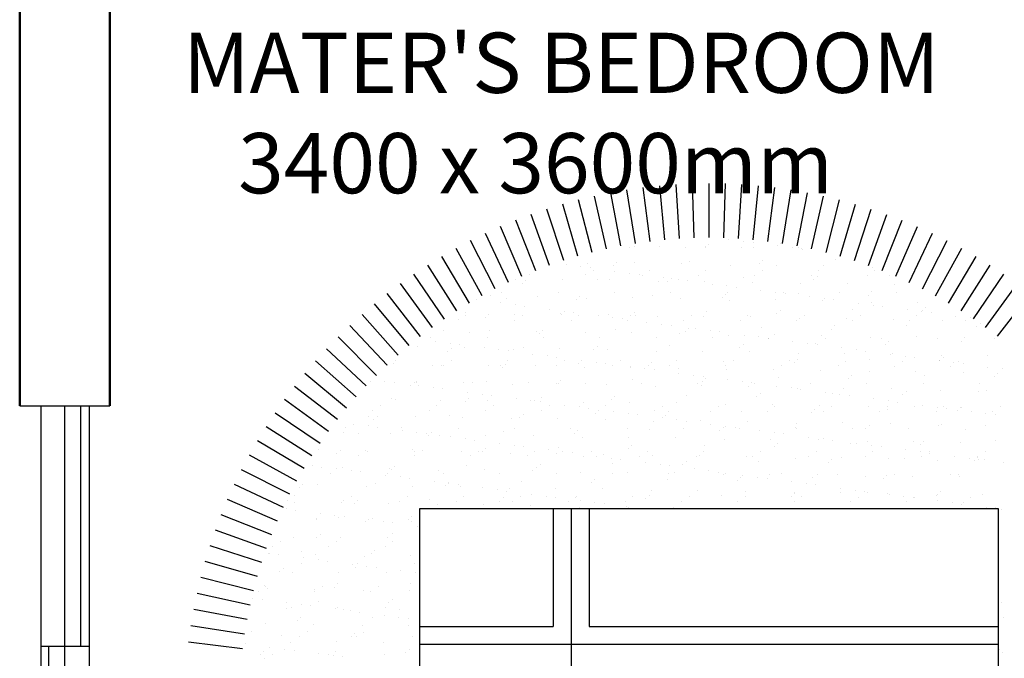
# Model space of a CAD drawing. Units: millimetres. Extents: x -857 to 54106, y -13666 to 13947.
# Tile 14 of 41: x 21020 to 23479, y 5837 to 7433. Entities that reach past the tile are written whole.
import ezdxf

# ---------------------------------------------------------------- set-up
doc = ezdxf.new("R2010")
doc.units = ezdxf.units.MM
for name, color, linetype, lineweight in [('A-AREA-IDEN', 3, 'Continuous', 18), ('A-FURN', 21, 'Continuous', 18), ('A-GLAZ', 4, 'Continuous', 25), ('A-WALL', 7, 'Continuous', 50)]:
    doc.layers.add(name, color=color, linetype=linetype, lineweight=lineweight)
for name, color, linetype in [('A-FRN', 11, 'Continuous'), ('A-HT', 15, 'Continuous'), ('L-HT', 1, 'Continuous')]:
    doc.layers.add(name, color=color, linetype=linetype)
doc.styles.get("Standard").update_dxf_attribs({"font": 'arial.ttf'})

# ---------------------------------------------------------------- blocks, each defined once
blk = doc.blocks.new('*X18')
at = {"color": 0}
for p, q in [((1.8017, 2.833), (1.8017, 2.833)), ((1.8783, 2.8364), (1.8783, 2.8364)), ((1.9044, 2.8399), (1.9044, 2.8399)), ((1.945, 2.8452), (1.945, 2.8452)), ((2.0018, 2.8313), (2.0018, 2.8313)), ((1.7428, 2.8186), (1.7428, 2.8186)), ((1.7438, 2.8187), (1.7438, 2.8187)), ((1.7537, 2.8227), (1.7537, 2.8227)), ((1.7698, 2.8221), (1.7698, 2.8221)), ((1.8104, 2.8275), (1.8104, 2.8275)), ((1.8778, 2.8235), (1.8778, 2.8235)), ((1.9094, 2.823), (1.9094, 2.823)), ((2.0087, 2.8252), (2.0087, 2.8252)), ((2.011, 2.8229), (2.011, 2.8229)), ((2.0652, 2.8233), (2.0652, 2.8233)), ((2.1366, 2.8246), (2.1366, 2.8246)), ((2.2048, 2.8269), (2.2048, 2.8269)), ((2.2209, 2.8236), (2.2209, 2.8236)), ((1.6514, 2.7891), (1.6514, 2.7891)), ((1.8515, 2.7874), (1.8515, 2.7874)), ((1.8607, 2.779), (1.8607, 2.779)), ((2.0545, 2.783), (2.0545, 2.783)), ((2.0763, 2.7783), (2.0763, 2.7783)), ((2.2072, 2.78), (2.2072, 2.78)), ((2.2546, 2.7813), (2.2546, 2.7813)), ((2.3351, 2.7793), (2.3351, 2.7793)), ((1.5414, 2.759), (1.5414, 2.759)), ((1.5474, 2.7675), (1.5474, 2.7675)), ((1.6825, 2.7724), (1.6825, 2.7724)), ((1.6971, 2.7593), (1.6971, 2.7593)), ((1.8133, 2.774), (1.8133, 2.774)), ((1.8528, 2.7596), (1.8528, 2.7596)), ((1.9412, 2.7734), (1.9412, 2.7734)), ((2.0085, 2.7599), (2.0085, 2.7599)), ((2.1643, 2.7602), (2.1643, 2.7602)), ((2.2196, 2.7519), (2.2196, 2.7519)), ((2.2603, 2.7573), (2.2603, 2.7573)), ((2.2638, 2.7728), (2.2638, 2.7728)), ((2.32, 2.7605), (2.32, 2.7605)), ((2.3282, 2.7662), (2.3282, 2.7662)), ((2.3542, 2.7696), (2.3542, 2.7696)), ((2.3949, 2.775), (2.3949, 2.775)), ((1.5011, 2.7453), (1.5011, 2.7453)), ((1.5625, 2.7456), (1.5625, 2.7456)), ((1.618, 2.7229), (1.618, 2.7229)), ((1.7012, 2.7435), (1.7012, 2.7435)), ((1.7104, 2.7351), (1.7104, 2.7351)), ((1.7182, 2.7459), (1.7182, 2.7459)), ((1.7459, 2.7223), (1.7459, 2.7223)), ((1.8739, 2.7462), (1.8739, 2.7462)), ((1.881, 2.7272), (1.881, 2.7272)), ((1.9042, 2.7391), (1.9042, 2.7391)), ((1.9911, 2.7218), (1.9911, 2.7218)), ((2.0118, 2.7288), (2.0118, 2.7288)), ((2.0296, 2.7465), (2.0296, 2.7465)), ((2.059, 2.7308), (2.059, 2.7308)), ((2.0851, 2.7342), (2.0851, 2.7342)), ((2.1043, 2.7374), (2.1043, 2.7374)), ((2.1135, 2.729), (2.1135, 2.729)), ((2.1257, 2.7395), (2.1257, 2.7395)), ((2.1397, 2.7282), (2.1397, 2.7282)), ((2.1853, 2.7467), (2.1853, 2.7467)), ((2.1936, 2.7485), (2.1936, 2.7485)), ((2.2748, 2.7331), (2.2748, 2.7331)), ((2.3073, 2.733), (2.3073, 2.733)), ((2.341, 2.747), (2.341, 2.747)), ((2.4057, 2.7348), (2.4057, 2.7348)), ((2.4967, 2.7473), (2.4967, 2.7473)), ((2.5074, 2.7313), (2.5074, 2.7313)), ((2.5166, 2.7228), (2.5166, 2.7228)), ((2.5336, 2.7341), (2.5336, 2.7341)), ((1.4827, 2.697), (1.4827, 2.697)), ((1.4871, 2.7212), (1.4871, 2.7212)), ((1.5509, 2.6997), (1.5509, 2.6997)), ((1.6384, 2.6973), (1.6384, 2.6973)), ((1.7539, 2.6952), (1.7539, 2.6952)), ((1.7899, 2.6953), (1.7899, 2.6953)), ((1.7941, 2.6975), (1.7941, 2.6975)), ((1.8159, 2.6988), (1.8159, 2.6988)), ((1.8565, 2.7041), (1.8565, 2.7041)), ((1.9244, 2.7131), (1.9244, 2.7131)), ((1.9498, 2.6978), (1.9498, 2.6978)), ((1.9505, 2.7165), (1.9505, 2.7165)), ((2.1055, 2.6981), (2.1055, 2.6981)), ((2.2612, 2.6984), (2.2612, 2.6984)), ((2.4169, 2.6987), (2.4169, 2.6987)), ((2.5727, 2.6989), (2.5727, 2.6989)), ((1.4227, 2.6718), (1.4227, 2.6718)), ((1.5506, 2.6712), (1.5506, 2.6712)), ((1.5601, 2.6912), (1.5601, 2.6912)), ((1.5873, 2.6687), (1.5873, 2.6687)), ((1.6553, 2.6776), (1.6553, 2.6776)), ((1.6813, 2.681), (1.6813, 2.681)), ((1.6856, 2.676), (1.6856, 2.676)), ((1.7219, 2.6864), (1.7219, 2.6864)), ((1.8165, 2.6777), (1.8165, 2.6777)), ((1.9444, 2.6771), (1.9444, 2.6771)), ((1.954, 2.6935), (1.954, 2.6935)), ((1.9632, 2.6851), (1.9632, 2.6851)), ((2.0794, 2.682), (2.0794, 2.682)), ((2.157, 2.6891), (2.157, 2.6891)), ((2.2103, 2.6836), (2.2103, 2.6836)), ((2.3382, 2.683), (2.3382, 2.683)), ((2.3571, 2.6874), (2.3571, 2.6874)), ((2.3663, 2.6789), (2.3663, 2.6789)), ((2.4733, 2.6879), (2.4733, 2.6879)), ((2.5601, 2.683), (2.5601, 2.683)), ((2.5756, 2.6693), (2.5756, 2.6693)), ((2.6042, 2.6895), (2.6042, 2.6895)), ((2.6435, 2.6783), (2.6435, 2.6783)), ((1.3861, 2.6422), (1.3861, 2.6422)), ((1.4006, 2.6558), (1.4006, 2.6558)), ((1.4098, 2.6473), (1.4098, 2.6473)), ((1.4121, 2.6456), (1.4121, 2.6456)), ((1.4528, 2.651), (1.4528, 2.651)), ((1.5207, 2.6599), (1.5207, 2.6599)), ((1.5467, 2.6633), (1.5467, 2.6633)), ((1.6036, 2.6513), (1.6036, 2.6513)), ((1.8037, 2.6496), (1.8037, 2.6496)), ((1.8129, 2.6412), (1.8129, 2.6412)), ((2.0067, 2.6452), (2.0067, 2.6452)), ((2.2068, 2.6435), (2.2068, 2.6435)), ((2.3743, 2.6428), (2.3743, 2.6428)), ((2.4003, 2.6462), (2.4003, 2.6462)), ((2.441, 2.6516), (2.441, 2.6516)), ((2.5089, 2.6605), (2.5089, 2.6605)), ((2.5349, 2.664), (2.5349, 2.664)), ((2.6718, 2.6427), (2.6718, 2.6427)), ((1.2775, 2.6279), (1.2775, 2.6279)), ((1.2915, 2.6198), (1.2915, 2.6198)), ((1.3182, 2.6332), (1.3182, 2.6332)), ((1.3552, 2.62), (1.3552, 2.62)), ((1.4261, 2.6336), (1.4261, 2.6336)), ((1.4472, 2.6201), (1.4472, 2.6201)), ((1.4903, 2.6249), (1.4903, 2.6249)), ((1.5818, 2.6338), (1.5818, 2.6338)), ((1.6029, 2.6204), (1.6029, 2.6204)), ((1.6212, 2.6266), (1.6212, 2.6266)), ((1.7375, 2.6341), (1.7375, 2.6341)), ((1.7491, 2.626), (1.7491, 2.626)), ((1.7586, 2.6207), (1.7586, 2.6207)), ((1.8841, 2.6308), (1.8841, 2.6308)), ((1.8932, 2.6344), (1.8932, 2.6344)), ((1.9143, 2.621), (1.9143, 2.621)), ((2.015, 2.6325), (2.015, 2.6325)), ((2.0489, 2.6347), (2.0489, 2.6347)), ((2.07, 2.6213), (2.07, 2.6213)), ((2.1429, 2.6319), (2.1429, 2.6319)), ((2.1718, 2.6162), (2.1718, 2.6162)), ((2.2046, 2.635), (2.2046, 2.635)), ((2.216, 2.635), (2.216, 2.635)), ((2.2257, 2.6215), (2.2257, 2.6215)), ((2.2397, 2.6251), (2.2397, 2.6251)), ((2.2657, 2.6285), (2.2657, 2.6285)), ((2.2779, 2.6367), (2.2779, 2.6367)), ((2.3064, 2.6339), (2.3064, 2.6339)), ((2.3603, 2.6352), (2.3603, 2.6352)), ((2.3814, 2.6218), (2.3814, 2.6218)), ((2.4088, 2.6384), (2.4088, 2.6384)), ((2.4098, 2.6391), (2.4098, 2.6391)), ((2.516, 2.6355), (2.516, 2.6355)), ((2.5367, 2.6378), (2.5367, 2.6378)), ((2.5371, 2.6221), (2.5371, 2.6221)), ((2.6099, 2.6374), (2.6099, 2.6374)), ((2.6191, 2.6289), (2.6191, 2.6289)), ((2.6718, 2.6358), (2.6718, 2.6358)), ((2.6928, 2.6224), (2.6928, 2.6224)), ((1.2503, 2.6119), (1.2503, 2.6119)), ((1.2595, 2.6034), (1.2595, 2.6034)), ((1.4533, 2.6075), (1.4533, 2.6075)), ((1.6534, 2.6057), (1.6534, 2.6057)), ((1.6626, 2.5973), (1.6626, 2.5973)), ((1.8564, 2.6013), (1.8564, 2.6013)), ((1.9705, 2.5897), (1.9705, 2.5897)), ((1.9966, 2.5931), (1.9966, 2.5931)), ((2.0372, 2.5984), (2.0372, 2.5984)), ((2.0565, 2.5996), (2.0565, 2.5996)), ((2.0657, 2.5912), (2.0657, 2.5912)), ((2.0826, 2.5856), (2.0826, 2.5856)), ((2.1051, 2.6074), (2.1051, 2.6074)), ((2.1312, 2.6108), (2.1312, 2.6108)), ((2.2135, 2.5873), (2.2135, 2.5873)), ((2.2595, 2.5952), (2.2595, 2.5952)), ((2.3414, 2.5867), (2.3414, 2.5867)), ((2.4595, 2.5935), (2.4595, 2.5935)), ((2.4764, 2.5915), (2.4764, 2.5915)), ((2.6073, 2.5932), (2.6073, 2.5932)), ((2.6626, 2.589), (2.6626, 2.589)), ((2.7352, 2.5926), (2.7352, 2.5926)), ((1.2117, 2.5712), (1.2117, 2.5712)), ((1.2949, 2.5738), (1.2949, 2.5738)), ((1.303, 2.5636), (1.303, 2.5636)), ((1.3674, 2.5715), (1.3674, 2.5715)), ((1.4258, 2.5754), (1.4258, 2.5754)), ((1.5031, 2.5619), (1.5031, 2.5619)), ((1.5231, 2.5718), (1.5231, 2.5718)), ((1.5537, 2.5748), (1.5537, 2.5748)), ((1.6788, 2.572), (1.6788, 2.572)), ((1.6888, 2.5797), (1.6888, 2.5797)), ((1.768, 2.563), (1.768, 2.563)), ((1.8196, 2.5814), (1.8196, 2.5814)), ((1.8345, 2.5723), (1.8345, 2.5723)), ((1.836, 2.5719), (1.836, 2.5719)), ((1.862, 2.5754), (1.862, 2.5754)), ((1.9026, 2.5807), (1.9026, 2.5807)), ((1.9475, 2.5807), (1.9475, 2.5807)), ((1.9902, 2.5726), (1.9902, 2.5726)), ((2.1459, 2.5729), (2.1459, 2.5729)), ((2.3016, 2.5732), (2.3016, 2.5732)), ((2.4573, 2.5735), (2.4573, 2.5735)), ((2.4688, 2.585), (2.4688, 2.585)), ((2.613, 2.5737), (2.613, 2.5737)), ((2.7156, 2.5583), (2.7156, 2.5583)), ((2.7563, 2.5636), (2.7563, 2.5636)), ((2.7687, 2.574), (2.7687, 2.574)), ((1.5123, 2.5534), (1.5123, 2.5534)), ((1.5668, 2.5365), (1.5668, 2.5365)), ((1.5928, 2.5399), (1.5928, 2.5399)), ((1.6334, 2.5453), (1.6334, 2.5453)), ((1.7014, 2.5542), (1.7014, 2.5542)), ((1.7061, 2.5574), (1.7061, 2.5574)), ((1.7274, 2.5577), (1.7274, 2.5577)), ((1.8873, 2.5345), (1.8873, 2.5345)), ((1.9061, 2.5557), (1.9061, 2.5557)), ((1.9154, 2.5473), (1.9154, 2.5473)), ((2.0181, 2.5361), (2.0181, 2.5361)), ((2.1092, 2.5513), (2.1092, 2.5513)), ((2.146, 2.5355), (2.146, 2.5355)), ((2.2811, 2.5404), (2.2811, 2.5404)), ((2.3092, 2.5496), (2.3092, 2.5496)), ((2.3185, 2.5411), (2.3185, 2.5411)), ((2.412, 2.5421), (2.412, 2.5421)), ((2.5123, 2.5452), (2.5123, 2.5452)), ((2.5399, 2.5415), (2.5399, 2.5415)), ((2.555, 2.5371), (2.555, 2.5371)), ((2.581, 2.5406), (2.581, 2.5406)), ((2.6217, 2.5459), (2.6217, 2.5459)), ((2.6749, 2.5463), (2.6749, 2.5463)), ((2.6896, 2.5549), (2.6896, 2.5549)), ((2.7123, 2.5434), (2.7123, 2.5434)), ((2.7216, 2.535), (2.7216, 2.535)), ((2.8058, 2.548), (2.8058, 2.548)), ((1.2305, 2.5243), (1.2305, 2.5243)), ((1.3108, 2.5081), (1.3108, 2.5081)), ((1.3236, 2.5045), (1.3236, 2.5045)), ((1.3527, 2.518), (1.3527, 2.518)), ((1.3584, 2.5237), (1.3584, 2.5237)), ((1.362, 2.5095), (1.362, 2.5095)), ((1.3643, 2.5098), (1.3643, 2.5098)), ((1.4322, 2.5188), (1.4322, 2.5188)), ((1.4582, 2.5222), (1.4582, 2.5222)), ((1.4665, 2.5083), (1.4665, 2.5083)), ((1.4934, 2.5286), (1.4934, 2.5286)), ((1.4989, 2.5276), (1.4989, 2.5276)), ((1.5558, 2.5136), (1.5558, 2.5136)), ((1.6222, 2.5086), (1.6222, 2.5086)), ((1.6243, 2.5302), (1.6243, 2.5302)), ((1.7522, 2.5296), (1.7522, 2.5296)), ((1.7558, 2.5118), (1.7558, 2.5118)), ((1.7779, 2.5089), (1.7779, 2.5089)), ((1.9336, 2.5092), (1.9336, 2.5092)), ((1.9589, 2.5074), (1.9589, 2.5074)), ((2.0893, 2.5095), (2.0893, 2.5095)), ((2.1589, 2.5057), (2.1589, 2.5057)), ((2.245, 2.5098), (2.245, 2.5098)), ((2.3118, 2.5051), (2.3118, 2.5051)), ((2.3525, 2.5105), (2.3525, 2.5105)), ((2.4007, 2.51), (2.4007, 2.51)), ((2.4204, 2.5194), (2.4204, 2.5194)), ((2.4464, 2.5229), (2.4464, 2.5229)), ((2.4871, 2.5282), (2.4871, 2.5282)), ((2.5564, 2.5103), (2.5564, 2.5103)), ((2.7121, 2.5106), (2.7121, 2.5106)), ((2.8678, 2.5109), (2.8678, 2.5109)), ((1.189, 2.4868), (1.189, 2.4868)), ((1.2297, 2.4921), (1.2297, 2.4921)), ((1.2976, 2.5011), (1.2976, 2.5011)), ((1.2981, 2.4774), (1.2981, 2.4774)), ((1.3319, 2.4946), (1.3319, 2.4946)), ((1.429, 2.4791), (1.429, 2.4791)), ((1.4876, 2.4949), (1.4876, 2.4949)), ((1.5569, 2.4785), (1.5569, 2.4785)), ((1.6433, 2.4952), (1.6433, 2.4952)), ((1.6919, 2.4833), (1.6919, 2.4833)), ((1.7651, 2.5034), (1.7651, 2.5034)), ((1.799, 2.4955), (1.799, 2.4955)), ((1.8228, 2.485), (1.8228, 2.485)), ((1.9507, 2.4844), (1.9507, 2.4844)), ((1.9547, 2.4958), (1.9547, 2.4958)), ((2.0857, 2.4893), (2.0857, 2.4893)), ((2.1104, 2.496), (2.1104, 2.496)), ((2.1512, 2.484), (2.1512, 2.484)), ((2.1682, 2.4973), (2.1682, 2.4973)), ((2.1773, 2.4874), (2.1773, 2.4874)), ((2.2166, 2.4909), (2.2166, 2.4909)), ((2.2179, 2.4928), (2.2179, 2.4928)), ((2.2661, 2.4963), (2.2661, 2.4963)), ((2.2858, 2.5017), (2.2858, 2.5017)), ((2.3445, 2.4903), (2.3445, 2.4903)), ((2.362, 2.5013), (2.362, 2.5013)), ((2.4218, 2.4966), (2.4218, 2.4966)), ((2.4796, 2.4952), (2.4796, 2.4952)), ((2.562, 2.4996), (2.562, 2.4996)), ((2.5712, 2.4911), (2.5712, 2.4911)), ((2.5775, 2.4969), (2.5775, 2.4969)), ((2.6104, 2.4969), (2.6104, 2.4969)), ((2.7332, 2.4972), (2.7332, 2.4972)), ((2.7384, 2.4962), (2.7384, 2.4962)), ((2.7651, 2.4951), (2.7651, 2.4951)), ((2.8734, 2.5011), (2.8734, 2.5011)), ((2.8889, 2.4975), (2.8889, 2.4975)), ((1.2024, 2.4741), (1.2024, 2.4741)), ((1.2117, 2.4657), (1.2117, 2.4657)), ((1.4055, 2.4697), (1.4055, 2.4697)), ((1.6055, 2.468), (1.6055, 2.468)), ((1.6148, 2.4595), (1.6148, 2.4595)), ((1.8086, 2.4635), (1.8086, 2.4635)), ((1.9081, 2.452), (1.9081, 2.452)), ((1.9487, 2.4573), (1.9487, 2.4573)), ((2.0086, 2.4618), (2.0086, 2.4618)), ((2.0166, 2.4663), (2.0166, 2.4663)), ((2.0178, 2.4534), (2.0178, 2.4534)), ((2.0427, 2.4697), (2.0427, 2.4697)), ((2.0833, 2.4751), (2.0833, 2.4751)), ((2.2117, 2.4574), (2.2117, 2.4574)), ((2.4117, 2.4557), (2.4117, 2.4557)), ((2.6147, 2.4513), (2.6147, 2.4513)), ((2.6781, 2.45), (2.6781, 2.45)), ((2.8089, 2.4516), (2.8089, 2.4516)), ((2.8148, 2.4495), (2.8148, 2.4495)), ((2.8963, 2.4526), (2.8963, 2.4526)), ((2.9368, 2.451), (2.9368, 2.451)), ((1.2336, 2.428), (1.2336, 2.428)), ((1.2521, 2.446), (1.2521, 2.446)), ((1.2552, 2.4258), (1.2552, 2.4258)), ((1.3615, 2.4273), (1.3615, 2.4273)), ((1.4078, 2.4463), (1.4078, 2.4463)), ((1.4552, 2.4241), (1.4552, 2.4241)), ((1.4966, 2.4322), (1.4966, 2.4322)), ((1.5635, 2.4466), (1.5635, 2.4466)), ((1.6275, 2.4339), (1.6275, 2.4339)), ((1.7192, 2.4468), (1.7192, 2.4468)), ((1.7475, 2.4308), (1.7475, 2.4308)), ((1.7554, 2.4333), (1.7554, 2.4333)), ((1.7735, 2.4343), (1.7735, 2.4343)), ((1.8141, 2.4396), (1.8141, 2.4396)), ((1.8749, 2.4471), (1.8749, 2.4471)), ((1.8821, 2.4486), (1.8821, 2.4486)), ((1.8904, 2.4381), (1.8904, 2.4381)), ((2.0213, 2.4398), (2.0213, 2.4398)), ((2.0306, 2.4474), (2.0306, 2.4474)), ((2.1492, 2.4392), (2.1492, 2.4392)), ((2.1863, 2.4477), (2.1863, 2.4477)), ((2.2842, 2.4441), (2.2842, 2.4441)), ((2.342, 2.448), (2.342, 2.448)), ((2.4151, 2.4457), (2.4151, 2.4457)), ((2.4209, 2.4472), (2.4209, 2.4472)), ((2.4977, 2.4483), (2.4977, 2.4483)), ((2.543, 2.4451), (2.543, 2.4451)), ((2.6534, 2.4485), (2.6534, 2.4485)), ((2.6678, 2.4225), (2.6678, 2.4225)), ((2.7357, 2.4315), (2.7357, 2.4315)), ((2.7617, 2.4349), (2.7617, 2.4349)), ((2.8024, 2.4403), (2.8024, 2.4403)), ((2.8091, 2.4488), (2.8091, 2.4488)), ((2.824, 2.4411), (2.824, 2.4411)), ((2.8703, 2.4492), (2.8703, 2.4492)), ((1.4644, 2.4156), (1.4644, 2.4156)), ((1.4783, 2.3954), (1.4783, 2.3954)), ((1.5043, 2.3988), (1.5043, 2.3988)), ((1.545, 2.4042), (1.545, 2.4042)), ((1.6129, 2.4131), (1.6129, 2.4131)), ((1.6389, 2.4165), (1.6389, 2.4165)), ((1.6582, 2.4197), (1.6582, 2.4197)), ((1.6795, 2.4219), (1.6795, 2.4219)), ((1.8583, 2.4179), (1.8583, 2.4179)), ((1.8675, 2.4095), (1.8675, 2.4095)), ((2.0613, 2.4135), (2.0613, 2.4135)), ((2.2614, 2.4118), (2.2614, 2.4118)), ((2.2706, 2.4033), (2.2706, 2.4033)), ((2.4644, 2.4074), (2.4644, 2.4074)), ((2.4665, 2.396), (2.4665, 2.396)), ((2.4827, 2.3988), (2.4827, 2.3988)), ((2.4925, 2.3995), (2.4925, 2.3995)), ((2.5332, 2.4048), (2.5332, 2.4048)), ((2.6011, 2.4138), (2.6011, 2.4138)), ((2.6136, 2.4005), (2.6136, 2.4005)), ((2.6271, 2.4172), (2.6271, 2.4172)), ((2.6645, 2.4057), (2.6645, 2.4057)), ((2.6737, 2.3972), (2.6737, 2.3972)), ((2.7415, 2.3999), (2.7415, 2.3999)), ((2.8675, 2.4012), (2.8675, 2.4012)), ((2.8765, 2.4048), (2.8765, 2.4048)), ((1.1954, 2.3826), (1.1954, 2.3826)), ((1.2165, 2.3691), (1.2165, 2.3691)), ((1.2758, 2.3687), (1.2758, 2.3687)), ((1.3012, 2.3811), (1.3012, 2.3811)), ((1.3049, 2.3802), (1.3049, 2.3802)), ((1.3141, 2.3717), (1.3141, 2.3717)), ((1.3437, 2.3777), (1.3437, 2.3777)), ((1.3512, 2.3829), (1.3512, 2.3829)), ((1.3697, 2.3811), (1.3697, 2.3811)), ((1.3722, 2.3694), (1.3722, 2.3694)), ((1.4104, 2.3865), (1.4104, 2.3865)), ((1.4321, 2.3828), (1.4321, 2.3828)), ((1.5069, 2.3831), (1.5069, 2.3831)), ((1.5079, 2.3758), (1.5079, 2.3758)), ((1.5279, 2.3697), (1.5279, 2.3697)), ((1.56, 2.3821), (1.56, 2.3821)), ((1.6626, 2.3834), (1.6626, 2.3834)), ((1.6837, 2.37), (1.6837, 2.37)), ((1.6951, 2.387), (1.6951, 2.387)), ((1.708, 2.374), (1.708, 2.374)), ((1.8183, 2.3837), (1.8183, 2.3837)), ((1.8259, 2.3887), (1.8259, 2.3887)), ((1.8394, 2.3703), (1.8394, 2.3703)), ((1.911, 2.3696), (1.911, 2.3696)), ((1.9538, 2.3881), (1.9538, 2.3881)), ((1.974, 2.384), (1.974, 2.384)), ((1.9951, 2.3706), (1.9951, 2.3706)), ((2.0889, 2.3929), (2.0889, 2.3929)), ((2.1111, 2.3679), (2.1111, 2.3679)), ((2.1297, 2.3843), (2.1297, 2.3843)), ((2.1508, 2.3708), (2.1508, 2.3708)), ((2.2198, 2.3946), (2.2198, 2.3946)), ((2.264, 2.3694), (2.264, 2.3694)), ((2.2854, 2.3846), (2.2854, 2.3846)), ((2.3065, 2.3711), (2.3065, 2.3711)), ((2.3319, 2.3783), (2.3319, 2.3783)), ((2.3477, 2.394), (2.3477, 2.394)), ((2.3579, 2.3817), (2.3579, 2.3817)), ((2.3986, 2.3871), (2.3986, 2.3871)), ((2.4411, 2.3848), (2.4411, 2.3848)), ((2.4622, 2.3714), (2.4622, 2.3714)), ((2.5968, 2.3851), (2.5968, 2.3851)), ((2.6179, 2.3717), (2.6179, 2.3717)), ((2.7525, 2.3854), (2.7525, 2.3854)), ((2.7736, 2.372), (2.7736, 2.372)), ((2.9082, 2.3857), (2.9082, 2.3857)), ((2.9293, 2.3723), (2.9293, 2.3723)), ((1.2091, 2.36), (1.2091, 2.36)), ((1.2351, 2.3634), (1.2351, 2.3634)), ((1.7172, 2.3656), (1.7172, 2.3656)), ((1.8936, 2.3418), (1.8936, 2.3418)), ((2.0244, 2.3435), (2.0244, 2.3435)), ((2.0627, 2.3429), (2.0627, 2.3429)), ((2.0888, 2.3463), (2.0888, 2.3463)), ((2.1203, 2.3595), (2.1203, 2.3595)), ((2.1294, 2.3517), (2.1294, 2.3517)), ((2.1523, 2.3429), (2.1523, 2.3429)), ((2.1973, 2.3606), (2.1973, 2.3606)), ((2.2234, 2.364), (2.2234, 2.364)), ((2.2874, 2.3477), (2.2874, 2.3477)), ((2.3141, 2.3635), (2.3141, 2.3635)), ((2.4183, 2.3494), (2.4183, 2.3494)), ((2.5142, 2.3618), (2.5142, 2.3618)), ((2.5234, 2.3533), (2.5234, 2.3533)), ((2.5462, 2.3488), (2.5462, 2.3488)), ((2.6812, 2.3536), (2.6812, 2.3536)), ((2.7172, 2.3573), (2.7172, 2.3573)), ((2.8121, 2.3553), (2.8121, 2.3553)), ((2.9173, 2.3556), (2.9173, 2.3556)), ((2.9265, 2.3472), (2.9265, 2.3472)), ((2.94, 2.3547), (2.94, 2.3547)), ((1.2368, 2.3316), (1.2368, 2.3316)), ((1.2924, 2.3208), (1.2924, 2.3208)), ((1.3576, 2.3319), (1.3576, 2.3319)), ((1.3647, 2.331), (1.3647, 2.331)), ((1.4481, 2.3211), (1.4481, 2.3211)), ((1.4997, 2.3359), (1.4997, 2.3359)), ((1.5577, 2.3302), (1.5577, 2.3302)), ((1.5669, 2.3217), (1.5669, 2.3217)), ((1.6038, 2.3214), (1.6038, 2.3214)), ((1.6306, 2.3375), (1.6306, 2.3375)), ((1.7585, 2.3369), (1.7585, 2.3369)), ((1.7596, 2.3216), (1.7596, 2.3216)), ((1.7607, 2.3257), (1.7607, 2.3257)), ((1.8602, 2.3162), (1.8602, 2.3162)), ((1.9153, 2.3219), (1.9153, 2.3219)), ((1.9282, 2.3252), (1.9282, 2.3252)), ((1.9542, 2.3286), (1.9542, 2.3286)), ((1.9608, 2.324), (1.9608, 2.324)), ((1.97, 2.3156), (1.97, 2.3156)), ((1.9948, 2.3339), (1.9948, 2.3339)), ((2.071, 2.3222), (2.071, 2.3222)), ((2.1638, 2.3196), (2.1638, 2.3196)), ((2.2267, 2.3225), (2.2267, 2.3225)), ((2.3639, 2.3179), (2.3639, 2.3179)), ((2.3824, 2.3228), (2.3824, 2.3228)), ((2.5381, 2.323), (2.5381, 2.323)), ((2.5669, 2.3135), (2.5669, 2.3135)), ((2.6938, 2.3233), (2.6938, 2.3233)), ((2.8485, 2.3169), (2.8485, 2.3169)), ((2.8495, 2.3236), (2.8495, 2.3236)), ((2.9164, 2.3258), (2.9164, 2.3258)), ((2.9424, 2.3292), (2.9424, 2.3292)), ((2.983, 2.3346), (2.983, 2.3346)), ((3.0052, 2.3239), (3.0052, 2.3239)), ((1.2073, 2.288), (1.2073, 2.288)), ((1.4074, 2.2863), (1.4074, 2.2863)), ((1.4353, 2.2864), (1.4353, 2.2864)), ((1.659, 2.2897), (1.659, 2.2897)), ((1.685, 2.2932), (1.685, 2.2932)), ((1.6982, 2.2907), (1.6982, 2.2907)), ((1.7256, 2.2985), (1.7256, 2.2985)), ((1.7936, 2.3074), (1.7936, 2.3074)), ((1.8196, 2.3109), (1.8196, 2.3109)), ((1.8291, 2.2923), (1.8291, 2.2923)), ((1.957, 2.2917), (1.957, 2.2917)), ((2.092, 2.2966), (2.092, 2.2966)), ((2.2229, 2.2983), (2.2229, 2.2983)), ((2.3508, 2.2976), (2.3508, 2.2976)), ((2.3731, 2.3094), (2.3731, 2.3094)), ((2.4859, 2.3025), (2.4859, 2.3025)), ((2.6167, 2.3042), (2.6167, 2.3042)), ((2.6472, 2.2904), (2.6472, 2.2904)), ((2.6732, 2.2938), (2.6732, 2.2938)), ((2.7139, 2.2992), (2.7139, 2.2992)), ((2.7447, 2.3036), (2.7447, 2.3036)), ((2.767, 2.3117), (2.767, 2.3117)), ((2.7762, 2.3033), (2.7762, 2.3033)), ((2.7818, 2.3081), (2.7818, 2.3081)), ((2.8078, 2.3115), (2.8078, 2.3115)), ((2.8797, 2.3084), (2.8797, 2.3084)), ((2.97, 2.3073), (2.97, 2.3073)), ((3.0106, 2.3101), (3.0106, 2.3101)), ((1.3044, 2.2847), (1.3044, 2.2847)), ((1.4166, 2.2778), (1.4166, 2.2778)), ((1.4565, 2.2631), (1.4565, 2.2631)), ((1.5244, 2.272), (1.5244, 2.272)), ((1.5504, 2.2754), (1.5504, 2.2754)), ((1.5632, 2.2858), (1.5632, 2.2858)), ((1.5911, 2.2808), (1.5911, 2.2808)), ((1.6104, 2.2819), (1.6104, 2.2819)), ((1.8105, 2.2801), (1.8105, 2.2801)), ((1.8197, 2.2717), (1.8197, 2.2717)), ((2.0135, 2.2757), (2.0135, 2.2757)), ((2.0144, 2.2588), (2.0144, 2.2588)), ((2.1701, 2.2591), (2.1701, 2.2591)), ((2.2136, 2.274), (2.2136, 2.274)), ((2.2228, 2.2656), (2.2228, 2.2656)), ((2.3258, 2.2594), (2.3258, 2.2594)), ((2.4166, 2.2696), (2.4166, 2.2696)), ((2.4447, 2.2637), (2.4447, 2.2637)), ((2.4815, 2.2596), (2.4815, 2.2596)), ((2.5126, 2.2727), (2.5126, 2.2727)), ((2.5386, 2.2761), (2.5386, 2.2761)), ((2.5793, 2.2814), (2.5793, 2.2814)), ((2.6167, 2.2679), (2.6167, 2.2679)), ((2.6259, 2.2594), (2.6259, 2.2594)), ((2.6372, 2.2599), (2.6372, 2.2599)), ((2.7929, 2.2602), (2.7929, 2.2602)), ((2.8152, 2.259), (2.8152, 2.259)), ((2.8197, 2.2634), (2.8197, 2.2634)), ((2.9486, 2.2605), (2.9486, 2.2605)), ((3.0198, 2.2617), (3.0198, 2.2617)), ((3.0782, 2.2632), (3.0782, 2.2632)), ((1.2358, 2.2574), (1.2358, 2.2574)), ((1.2399, 2.2353), (1.2399, 2.2353)), ((1.2552, 2.2366), (1.2552, 2.2366)), ((1.2569, 2.2439), (1.2569, 2.2439)), ((1.2571, 2.2424), (1.2571, 2.2424)), ((1.2663, 2.234), (1.2663, 2.234)), ((1.2812, 2.24), (1.2812, 2.24)), ((1.3219, 2.2453), (1.3219, 2.2453)), ((1.3678, 2.2347), (1.3678, 2.2347)), ((1.3898, 2.2543), (1.3898, 2.2543)), ((1.3915, 2.2577), (1.3915, 2.2577)), ((1.4126, 2.2442), (1.4126, 2.2442)), ((1.4158, 2.2577), (1.4158, 2.2577)), ((1.4601, 2.238), (1.4601, 2.238)), ((1.5029, 2.2395), (1.5029, 2.2395)), ((1.5472, 2.2579), (1.5472, 2.2579)), ((1.5683, 2.2445), (1.5683, 2.2445)), ((1.6338, 2.2412), (1.6338, 2.2412)), ((1.6602, 2.2363), (1.6602, 2.2363)), ((1.7029, 2.2582), (1.7029, 2.2582)), ((1.724, 2.2448), (1.724, 2.2448)), ((1.7617, 2.2406), (1.7617, 2.2406)), ((1.8587, 2.2585), (1.8587, 2.2585)), ((1.8632, 2.2318), (1.8632, 2.2318)), ((1.8797, 2.2451), (1.8797, 2.2451)), ((1.8967, 2.2455), (1.8967, 2.2455)), ((2.0276, 2.2471), (2.0276, 2.2471)), ((2.0354, 2.2454), (2.0354, 2.2454)), ((2.1555, 2.2465), (2.1555, 2.2465)), ((2.1912, 2.2456), (2.1912, 2.2456)), ((2.2434, 2.2372), (2.2434, 2.2372)), ((2.2695, 2.2406), (2.2695, 2.2406)), ((2.2905, 2.2514), (2.2905, 2.2514)), ((2.3101, 2.246), (2.3101, 2.246)), ((2.3469, 2.2459), (2.3469, 2.2459)), ((2.378, 2.2549), (2.378, 2.2549)), ((2.404, 2.2584), (2.404, 2.2584)), ((2.4214, 2.253), (2.4214, 2.253)), ((2.5026, 2.2462), (2.5026, 2.2462)), ((2.5493, 2.2524), (2.5493, 2.2524)), ((2.6583, 2.2465), (2.6583, 2.2465)), ((2.6844, 2.2573), (2.6844, 2.2573)), ((2.814, 2.2468), (2.814, 2.2468)), ((2.9431, 2.2584), (2.9431, 2.2584)), ((2.9697, 2.2471), (2.9697, 2.2471)), ((3.029, 2.2533), (3.029, 2.2533)), ((1.1873, 2.2276), (1.1873, 2.2276)), ((1.6694, 2.2278), (1.6694, 2.2278)), ((2.0003, 2.2052), (2.0003, 2.2052)), ((2.0409, 2.2106), (2.0409, 2.2106)), ((2.0633, 2.2301), (2.0633, 2.2301)), ((2.0725, 2.2217), (2.0725, 2.2217)), ((2.1088, 2.2195), (2.1088, 2.2195)), ((2.1349, 2.2229), (2.1349, 2.2229)), ((2.1755, 2.2283), (2.1755, 2.2283)), ((2.2663, 2.2257), (2.2663, 2.2257)), ((2.4664, 2.224), (2.4664, 2.224)), ((2.4756, 2.2155), (2.4756, 2.2155)), ((2.489, 2.2062), (2.489, 2.2062)), ((2.6199, 2.2078), (2.6199, 2.2078)), ((2.6694, 2.2196), (2.6694, 2.2196)), ((2.7478, 2.2072), (2.7478, 2.2072)), ((2.8695, 2.2178), (2.8695, 2.2178)), ((2.8787, 2.2094), (2.8787, 2.2094)), ((2.8828, 2.2121), (2.8828, 2.2121)), ((2.9885, 2.2058), (2.9885, 2.2058)), ((3.0137, 2.2138), (3.0137, 2.2138)), ((3.0291, 2.2112), (3.0291, 2.2112)), ((3.0725, 2.2134), (3.0725, 2.2134)), ((3.0971, 2.2201), (3.0971, 2.2201)), ((1.3075, 2.1884), (1.3075, 2.1884)), ((1.3098, 2.1941), (1.3098, 2.1941)), ((1.3328, 2.1956), (1.3328, 2.1956)), ((1.4384, 2.1901), (1.4384, 2.1901)), ((1.4885, 2.1959), (1.4885, 2.1959)), ((1.5099, 2.1924), (1.5099, 2.1924)), ((1.5191, 2.1839), (1.5191, 2.1839)), ((1.5663, 2.1895), (1.5663, 2.1895)), ((1.6442, 2.1961), (1.6442, 2.1961)), ((1.7014, 2.1943), (1.7014, 2.1943)), ((1.7129, 2.188), (1.7129, 2.188)), ((1.7999, 2.1964), (1.7999, 2.1964)), ((1.8322, 2.196), (1.8322, 2.196)), ((1.8397, 2.1841), (1.8397, 2.1841)), ((1.8657, 2.1875), (1.8657, 2.1875)), ((1.9063, 2.1928), (1.9063, 2.1928)), ((1.913, 2.1862), (1.913, 2.1862)), ((1.9222, 2.1778), (1.9222, 2.1778)), ((1.9556, 2.1967), (1.9556, 2.1967)), ((1.9601, 2.1954), (1.9601, 2.1954)), ((1.9743, 2.2018), (1.9743, 2.2018)), ((2.0952, 2.2002), (2.0952, 2.2002)), ((2.1114, 2.197), (2.1114, 2.197)), ((2.116, 2.1818), (2.116, 2.1818)), ((2.2261, 2.2019), (2.2261, 2.2019)), ((2.2671, 2.1973), (2.2671, 2.1973)), ((2.3161, 2.1801), (2.3161, 2.1801)), ((2.354, 2.2013), (2.354, 2.2013)), ((2.4228, 2.1976), (2.4228, 2.1976)), ((2.5785, 2.1978), (2.5785, 2.1978)), ((2.7342, 2.1981), (2.7342, 2.1981)), ((2.8279, 2.1847), (2.8279, 2.1847)), ((2.8539, 2.1881), (2.8539, 2.1881)), ((2.8899, 2.1984), (2.8899, 2.1984)), ((2.8946, 2.1935), (2.8946, 2.1935)), ((2.9625, 2.2024), (2.9625, 2.2024)), ((3.0456, 2.1987), (3.0456, 2.1987)), ((1.5965, 2.152), (1.5965, 2.152)), ((1.6372, 2.1574), (1.6372, 2.1574)), ((1.7051, 2.1663), (1.7051, 2.1663)), ((1.7311, 2.1698), (1.7311, 2.1698)), ((1.7717, 2.1751), (1.7717, 2.1751)), ((2.0307, 2.1508), (2.0307, 2.1508)), ((2.1586, 2.1502), (2.1586, 2.1502)), ((2.2937, 2.155), (2.2937, 2.155)), ((2.3253, 2.1717), (2.3253, 2.1717)), ((2.4246, 2.1567), (2.4246, 2.1567)), ((2.5191, 2.1757), (2.5191, 2.1757)), ((2.5525, 2.1561), (2.5525, 2.1561)), ((2.5847, 2.1527), (2.5847, 2.1527)), ((2.6254, 2.158), (2.6254, 2.158)), ((2.6875, 2.161), (2.6875, 2.161)), ((2.6933, 2.167), (2.6933, 2.167)), ((2.7192, 2.174), (2.7192, 2.174)), ((2.7193, 2.1704), (2.7193, 2.1704)), ((2.7284, 2.1655), (2.7284, 2.1655)), ((2.76, 2.1758), (2.76, 2.1758)), ((2.8184, 2.1626), (2.8184, 2.1626)), ((2.9222, 2.1695), (2.9222, 2.1695)), ((2.9463, 2.162), (2.9463, 2.162)), ((3.0813, 2.1669), (3.0813, 2.1669)), ((3.1223, 2.1678), (3.1223, 2.1678)), ((3.1315, 2.1594), (3.1315, 2.1594)), ((1.2431, 2.1389), (1.2431, 2.1389)), ((1.2762, 2.1322), (1.2762, 2.1322)), ((1.3596, 2.1485), (1.3596, 2.1485)), ((1.3688, 2.14), (1.3688, 2.14)), ((1.371, 2.1383), (1.371, 2.1383)), ((1.4319, 2.1324), (1.4319, 2.1324)), ((1.4359, 2.1309), (1.4359, 2.1309)), ((1.4619, 2.1343), (1.4619, 2.1343)), ((1.5026, 2.1397), (1.5026, 2.1397)), ((1.506, 2.1432), (1.506, 2.1432)), ((1.5626, 2.1441), (1.5626, 2.1441)), ((1.5705, 2.1486), (1.5705, 2.1486)), ((1.5876, 2.1327), (1.5876, 2.1327)), ((1.6369, 2.1449), (1.6369, 2.1449)), ((1.7433, 2.133), (1.7433, 2.133)), ((1.7627, 2.1424), (1.7627, 2.1424)), ((1.7648, 2.1442), (1.7648, 2.1442)), ((1.7719, 2.1339), (1.7719, 2.1339)), ((1.899, 2.1333), (1.899, 2.1333)), ((1.8999, 2.1491), (1.8999, 2.1491)), ((1.9657, 2.1379), (1.9657, 2.1379)), ((2.0547, 2.1336), (2.0547, 2.1336)), ((2.1658, 2.1362), (2.1658, 2.1362)), ((2.175, 2.1278), (2.175, 2.1278)), ((2.2105, 2.1339), (2.2105, 2.1339)), ((2.3662, 2.1341), (2.3662, 2.1341)), ((2.3688, 2.1318), (2.3688, 2.1318)), ((2.4241, 2.1315), (2.4241, 2.1315)), ((2.4501, 2.135), (2.4501, 2.135)), ((2.4908, 2.1403), (2.4908, 2.1403)), ((2.5219, 2.1344), (2.5219, 2.1344)), ((2.5587, 2.1493), (2.5587, 2.1493)), ((2.5689, 2.1301), (2.5689, 2.1301)), ((2.6776, 2.1347), (2.6776, 2.1347)), ((2.7719, 2.1257), (2.7719, 2.1257)), ((2.8333, 2.135), (2.8333, 2.135)), ((2.972, 2.1239), (2.972, 2.1239)), ((2.989, 2.1353), (2.989, 2.1353)), ((3.1447, 2.1356), (3.1447, 2.1356)), ((1.1927, 2.0989), (1.1927, 2.0989)), ((1.2093, 2.1046), (1.2093, 2.1046)), ((1.2334, 2.1042), (1.2334, 2.1042)), ((1.2973, 2.1187), (1.2973, 2.1187)), ((1.3013, 2.1132), (1.3013, 2.1132)), ((1.3273, 2.1166), (1.3273, 2.1166)), ((1.368, 2.122), (1.368, 2.122)), ((1.4123, 2.1002), (1.4123, 2.1002)), ((1.453, 2.119), (1.453, 2.119)), ((1.6087, 2.1193), (1.6087, 2.1193)), ((1.7644, 2.1196), (1.7644, 2.1196)), ((1.9201, 2.1199), (1.9201, 2.1199)), ((2.0758, 2.1201), (2.0758, 2.1201)), ((2.0983, 2.1039), (2.0983, 2.1039)), ((2.2216, 2.1049), (2.2216, 2.1049)), ((2.2292, 2.1056), (2.2292, 2.1056)), ((2.2315, 2.1204), (2.2315, 2.1204)), ((2.2895, 2.1138), (2.2895, 2.1138)), ((2.3156, 2.1173), (2.3156, 2.1173)), ((2.3562, 2.1226), (2.3562, 2.1226)), ((2.3571, 2.105), (2.3571, 2.105)), ((2.3872, 2.1207), (2.3872, 2.1207)), ((2.4922, 2.1098), (2.4922, 2.1098)), ((2.5429, 2.121), (2.5429, 2.121)), ((2.5781, 2.1216), (2.5781, 2.1216)), ((2.623, 2.1115), (2.623, 2.1115)), ((2.6987, 2.1213), (2.6987, 2.1213)), ((2.751, 2.1109), (2.751, 2.1109)), ((2.8544, 2.1216), (2.8544, 2.1216)), ((2.886, 2.1157), (2.886, 2.1157)), ((2.9812, 2.1155), (2.9812, 2.1155)), ((3.0101, 2.1218), (3.0101, 2.1218)), ((3.0169, 2.1174), (3.0169, 2.1174)), ((3.1432, 2.0968), (3.1432, 2.0968)), ((3.1448, 2.1168), (3.1448, 2.1168)), ((3.1658, 2.1221), (3.1658, 2.1221)), ((3.1692, 2.1002), (3.1692, 2.1002)), ((2.8216, 2.08), (2.8216, 2.08)), ((2.8309, 2.0716), (2.8309, 2.0716)), ((2.9303, 2.0732), (2.9303, 2.0732)), ((2.9407, 2.0701), (2.9407, 2.0701)), ((3.0086, 2.079), (3.0086, 2.079)), ((3.0247, 2.0756), (3.0247, 2.0756)), ((3.0346, 2.0825), (3.0346, 2.0825)), ((3.0752, 2.0878), (3.0752, 2.0878)), ((3.0845, 2.0705), (3.0845, 2.0705)), ((3.086, 2.0735), (3.086, 2.0735)), ((2.8061, 2.0524), (2.8061, 2.0524)), ((2.8215, 2.0663), (2.8215, 2.0663)), ((2.874, 2.0613), (2.874, 2.0613)), ((2.9, 2.0647), (2.9, 2.0647)), ((2.9494, 2.0657), (2.9494, 2.0657)), ((2.8744, 2.0317), (2.8744, 2.0317)), ((2.8891, 2.0194), (2.8891, 2.0194)), ((3.02, 2.0211), (3.02, 2.0211)), ((3.0744, 2.03), (3.0744, 2.03)), ((3.0837, 2.0216), (3.0837, 2.0216)), ((3.1479, 2.0205), (3.1479, 2.0205)), ((2.8737, 2.0098), (2.8737, 2.0098)), ((2.8947, 1.9964), (2.8947, 1.9964)), ((3.0294, 2.0101), (3.0294, 2.0101)), ((3.0505, 1.9966), (3.0505, 1.9966)), ((3.1851, 2.0104), (3.1851, 2.0104)), ((3.2062, 1.9969), (3.2062, 1.9969)), ((2.8247, 1.9699), (2.8247, 1.9699)), ((2.9241, 1.9861), (2.9241, 1.9861)), ((2.9333, 1.9777), (2.9333, 1.9777)), ((2.9526, 1.9693), (2.9526, 1.9693)), ((3.0876, 1.9742), (3.0876, 1.9742)), ((3.1213, 1.9644), (3.1213, 1.9644)), ((3.1272, 1.9817), (3.1272, 1.9817)), ((3.1893, 1.9734), (3.1893, 1.9734)), ((3.2153, 1.9768), (3.2153, 1.9768)), ((3.2185, 1.9759), (3.2185, 1.9759)), ((2.8149, 1.9477), (2.8149, 1.9477)), ((2.9201, 1.9379), (2.9201, 1.9379)), ((2.9461, 1.9414), (2.9461, 1.9414)), ((2.9707, 1.948), (2.9707, 1.948)), ((2.9768, 1.9378), (2.9768, 1.9378)), ((2.9868, 1.9467), (2.9868, 1.9467)), ((3.0547, 1.9556), (3.0547, 1.9556)), ((3.0807, 1.9591), (3.0807, 1.9591)), ((3.1264, 1.9483), (3.1264, 1.9483)), ((3.1769, 1.9361), (3.1769, 1.9361)), ((2.8115, 1.9236), (2.8115, 1.9236)), ((2.8522, 1.929), (2.8522, 1.929)), ((2.8923, 1.9231), (2.8923, 1.9231)), ((3.0232, 1.9247), (3.0232, 1.9247)), ((3.1511, 1.9241), (3.1511, 1.9241)), ((3.1861, 1.9277), (3.1861, 1.9277)), ((2.8265, 1.894), (2.8265, 1.894)), ((2.914, 1.8846), (2.914, 1.8846)), ((3.0266, 1.8922), (3.0266, 1.8922)), ((3.0358, 1.8838), (3.0358, 1.8838)), ((3.0697, 1.8849), (3.0697, 1.8849)), ((3.0908, 1.8779), (3.0908, 1.8779)), ((3.2217, 1.8795), (3.2217, 1.8795)), ((3.2255, 1.8852), (3.2255, 1.8852)), ((3.2296, 1.8878), (3.2296, 1.8878)), ((2.8278, 1.8736), (2.8278, 1.8736)), ((2.9351, 1.8712), (2.9351, 1.8712)), ((2.9557, 1.873), (2.9557, 1.873)), ((3.0908, 1.8714), (3.0908, 1.8714)), ((3.2465, 1.8717), (3.2465, 1.8717)), ((3.2614, 1.8534), (3.2614, 1.8534)), ((1.191, 1.8397), (1.191, 1.8397)), ((2.8763, 1.8484), (2.8763, 1.8484)), ((2.8855, 1.8399), (2.8855, 1.8399)), ((2.8954, 1.8267), (2.8954, 1.8267)), ((3.0263, 1.8284), (3.0263, 1.8284)), ((3.0329, 1.8233), (3.0329, 1.8233)), ((3.0793, 1.8439), (3.0793, 1.8439)), ((3.1008, 1.8323), (3.1008, 1.8323)), ((3.1268, 1.8357), (3.1268, 1.8357)), ((3.1542, 1.8278), (3.1542, 1.8278)), ((3.1674, 1.841), (3.1674, 1.841)), ((3.2354, 1.85), (3.2354, 1.85)), ((1.1851, 1.7982), (1.1851, 1.7982)), ((2.8316, 1.7968), (2.8316, 1.7968)), ((2.8553, 1.8225), (2.8553, 1.8225)), ((2.8576, 1.8002), (2.8576, 1.8002)), ((2.8983, 1.8056), (2.8983, 1.8056)), ((2.929, 1.8), (2.929, 1.8)), ((2.9662, 1.8145), (2.9662, 1.8145)), ((2.9922, 1.818), (2.9922, 1.818)), ((3.011, 1.8228), (3.011, 1.8228)), ((3.1291, 1.7983), (3.1291, 1.7983)), ((3.1667, 1.8231), (3.1667, 1.8231)), ((2.831, 1.7773), (2.831, 1.7773)), ((2.9589, 1.7766), (2.9589, 1.7766)), ((3.0939, 1.7815), (3.0939, 1.7815)), ((3.1383, 1.7899), (3.1383, 1.7899)), ((3.2248, 1.7832), (3.2248, 1.7832)), ((2.8198, 1.7457), (2.8198, 1.7457)), ((2.9544, 1.7594), (2.9544, 1.7594)), ((2.9755, 1.7459), (2.9755, 1.7459)), ((2.9788, 1.7544), (2.9788, 1.7544)), ((2.988, 1.746), (2.988, 1.746)), ((3.1101, 1.7597), (3.1101, 1.7597)), ((3.1312, 1.7462), (3.1312, 1.7462)), ((3.1818, 1.75), (3.1818, 1.75)), ((3.2658, 1.7599), (3.2658, 1.7599)), ((2.8986, 1.7304), (2.8986, 1.7304)), ((3.0295, 1.7321), (3.0295, 1.7321)), ((3.1574, 1.7314), (3.1574, 1.7314)), ((3.2135, 1.7176), (3.2135, 1.7176)), ((3.2815, 1.7266), (3.2815, 1.7266)), ((1.1882, 1.7018), (1.1882, 1.7018)), ((1.1965, 1.711), (1.1965, 1.711)), ((2.8285, 1.7106), (2.8285, 1.7106)), ((2.8377, 1.7021), (2.8377, 1.7021)), ((2.8957, 1.6973), (2.8957, 1.6973)), ((3.0123, 1.6911), (3.0123, 1.6911)), ((3.0315, 1.7061), (3.0315, 1.7061)), ((3.0383, 1.6946), (3.0383, 1.6946)), ((3.0514, 1.6976), (3.0514, 1.6976)), ((3.079, 1.6999), (3.079, 1.6999)), ((3.1469, 1.7089), (3.1469, 1.7089)), ((3.1729, 1.7123), (3.1729, 1.7123)), ((3.2071, 1.6979), (3.2071, 1.6979)), ((3.2316, 1.7044), (3.2316, 1.7044)), ((3.2408, 1.696), (3.2408, 1.696)), ((3.228, 1.6868), (3.228, 1.6868))]:
    blk.add_line(p, q, dxfattribs=at)
blk = doc.blocks.new('A$C6796526C')
at = {"layer": 'A-FRN'}
blk.add_lwpolyline([(0.65, 2.8), (0.65, 0.9), (2.25, 0.9), (2.25, 2.8)], dxfattribs=at)
at = {"layer": 'A-HT'}
for p, q in [((2.7397, 1.2871), (2.8886, 1.2683)), ((2.734, 1.2466), (2.8821, 1.2232)), ((2.727, 1.2064), (2.8743, 1.1783)), ((2.7187, 1.1664), (2.8651, 1.1337)), ((2.7092, 1.1267), (2.8544, 1.0894)), ((2.6984, 1.0873), (2.8424, 1.0455)), ((2.6864, 1.0483), (2.829, 1.0019)), ((2.6731, 1.0096), (2.8143, 0.9588)), ((2.6587, 0.9714), (2.7982, 0.9162)), ((2.6431, 0.9337), (2.7807, 0.8741)), ((2.6263, 0.8965), (2.762, 0.8326)), ((2.6083, 0.8598), (2.742, 0.7917)), ((2.5892, 0.8237), (2.7206, 0.7515)), ((2.569, 0.7882), (2.6981, 0.7119)), ((2.5476, 0.7534), (2.6743, 0.6731)), ((2.5252, 0.7193), (2.6493, 0.635)), ((2.5017, 0.6859), (2.6231, 0.5977)), ((2.4772, 0.6532), (2.5957, 0.5613)), ((2.4517, 0.6213), (2.5672, 0.5257)), ((2.4251, 0.5903), (2.5377, 0.4911)), ((2.3977, 0.5601), (2.507, 0.4574)), ((2.3692, 0.5308), (2.4753, 0.4247)), ((2.3399, 0.5023), (2.4426, 0.393)), ((2.3097, 0.4749), (2.4089, 0.3623)), ((2.2787, 0.4483), (2.3743, 0.3328)), ((0.6532, 0.4228), (0.5613, 0.3043)), ((2.2474, 0.423), (2.3394, 0.3045)), ((0.6859, 0.3983), (0.5977, 0.2769)), ((2.2148, 0.3985), (2.303, 0.2772)), ((0.7193, 0.3748), (0.635, 0.2507)), ((2.1814, 0.375), (2.2657, 0.251)), ((0.7534, 0.3524), (0.6731, 0.2257)), ((0.7882, 0.331), (0.7119, 0.2019)), ((2.1124, 0.3313), (2.1888, 0.2022)), ((2.1472, 0.3526), (2.2276, 0.226)), ((0.8237, 0.3108), (0.7515, 0.1794)), ((2.0769, 0.311), (2.1492, 0.1796)), ((0.8598, 0.2917), (0.7917, 0.158)), ((0.8965, 0.2737), (0.8326, 0.138)), ((2.0042, 0.274), (2.068, 0.1382)), ((2.0409, 0.2919), (2.109, 0.1583)), ((0.9337, 0.2569), (0.8741, 0.1193)), ((1.967, 0.2572), (2.0265, 0.1195)), ((0.9714, 0.2413), (0.9162, 0.1018)), ((1.0096, 0.2269), (0.9588, 0.0857)), ((1.891, 0.2271), (1.9418, 0.086)), ((1.9292, 0.2415), (1.9844, 0.1021)), ((1.0483, 0.2136), (1.0019, 0.071)), ((1.0873, 0.2016), (1.0455, 0.0576)), ((1.1267, 0.1908), (1.0894, 0.0456)), ((1.7733, 0.1908), (1.8106, 0.0456)), ((1.8127, 0.2016), (1.8545, 0.0576)), ((1.8517, 0.2136), (1.8981, 0.071)), ((1.1664, 0.1813), (1.1337, 0.0349)), ((1.2064, 0.173), (1.1783, 0.0257)), ((1.2466, 0.166), (1.2232, 0.0179)), ((1.6534, 0.166), (1.6768, 0.0179)), ((1.6936, 0.173), (1.7217, 0.0257)), ((1.7336, 0.1813), (1.7663, 0.0349)), ((1.2871, 0.1603), (1.2683, 0.0114)), ((1.3277, 0.1558), (1.3135, 0.0064)), ((1.3684, 0.1526), (1.359, 0.0029)), ((1.4092, 0.1506), (1.4045, 0.0007)), ((1.45, 0.15), (1.45, 0)), ((1.4908, 0.1506), (1.4955, 0.0007)), ((1.5316, 0.1526), (1.541, 0.0029)), ((1.5723, 0.1558), (1.5865, 0.0064)), ((1.6129, 0.1603), (1.6317, 0.0114))]:
    blk.add_line(p, q, dxfattribs=at)
at = {"layer": 'L-HT'}
for p, q in [((1.8309, 0.9), (1.8309, 2.2094)), ((0.65, 1.2749), (2.25, 1.2749)), ((1.7809, 1.2249), (0.65, 1.2249)), ((1.7809, 0.9), (1.7809, 1.2249)), ((1.8809, 0.9), (1.8809, 1.2249)), ((2.25, 1.2249), (1.8809, 1.2249))]:
    blk.add_line(p, q, dxfattribs=at)
at = {"layer": 'A-HT', "extrusion": (0, 0, -1), "zscale": -1, "rotation": 180}
blk.add_blockref('*X18', (0.55, 3), dxfattribs=at)
blk = doc.blocks.new('WIN-1200')
for p, q in [((9371.3, 11750.2), (10571.3, 11750.2)), ((9371.3, 11731.7), (9971.3, 11731.7)), ((9971.3, 11750.2), (9971.3, 11630.7)), ((9371.3, 11691.7), (10571.3, 11691.7)), ((9971.3, 11651.7), (10571.3, 11651.7)), ((10571.3, 11630.7), (9371.3, 11630.7))]:
    blk.add_line(p, q)
for points in [[(9371.3, 11579.2), (9371.3, 11804.2)], [(10571.3, 11804.2), (10571.3, 11579.2)]]:
    blk.add_lwpolyline(points)

msp = doc.modelspace()

# ---------------------------------------------------------------- linework, layer by layer
at = {"layer": 'A-WALL'}
msp.add_line((21245.079, 6467.586), (21245.079, 7729.231), dxfattribs=at)
msp.add_lwpolyline([(21020.079, 6467.586), (21020.079, 8304.231)], dxfattribs=at)

# ---------------------------------------------------------------- block references
at = {"layer": 'A-FURN', "xscale": 903.6084929786902, "yscale": 903.6084929786902, "zscale": 903.6084929786902, "rotation": 179.9999999999989}
msp.add_blockref('A$C6796526C', (24051.97, 7023.692), dxfattribs=at)
at = {"layer": 'A-GLAZ', "rotation": 90.00000000000063}
msp.add_blockref('WIN-1200', (32824.31, -4103.754), dxfattribs=at)

# ---------------------------------------------------------------- texts
at = {"layer": 'A-AREA-IDEN', "insert": (21427.662, 7400.355), "char_height": 150.48461, "attachment_point": 1}
msp.add_mtext_dynamic_manual_height_columns("\\pxt0;MATER'S BEDROOM\\P   3400 x 3600mm", width=2554.22693, gutter_width=18810.576, heights=[2595.835], dxfattribs=at)

doc.saveas('drawing.dxf')
